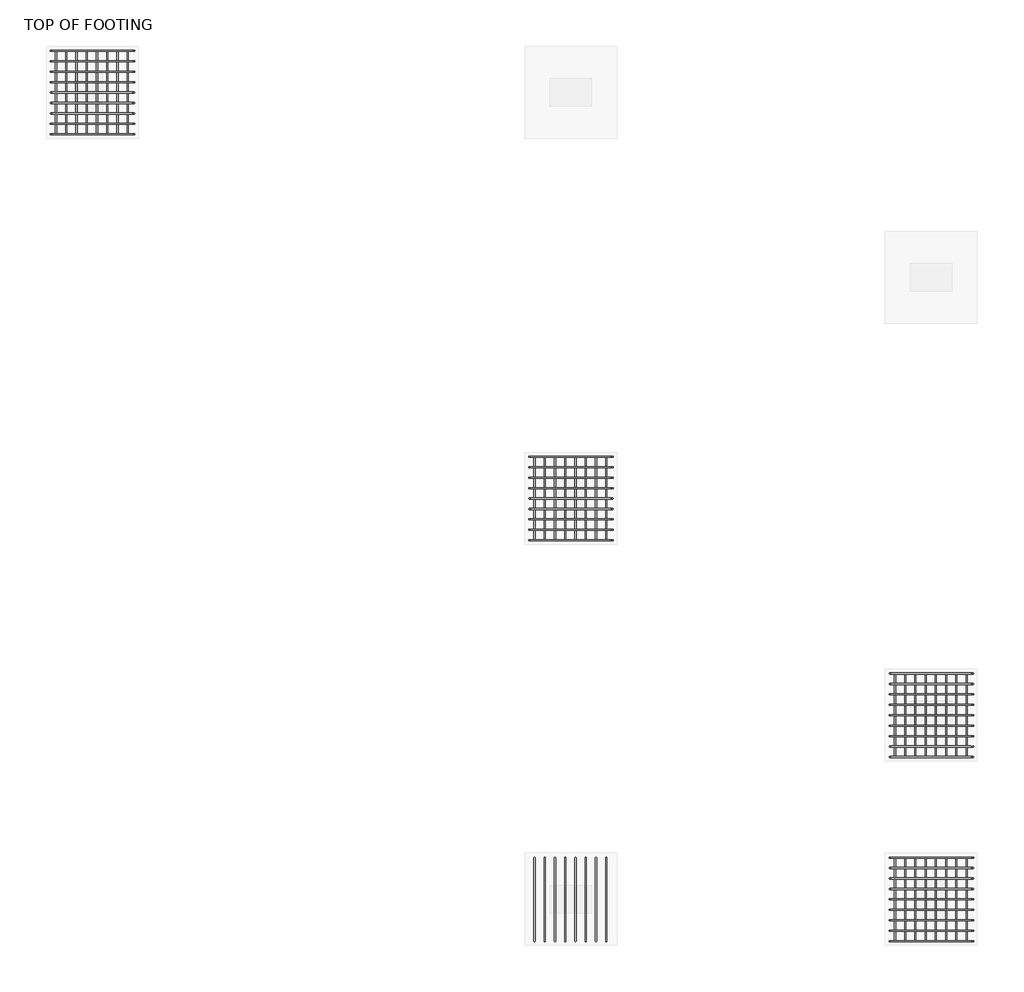
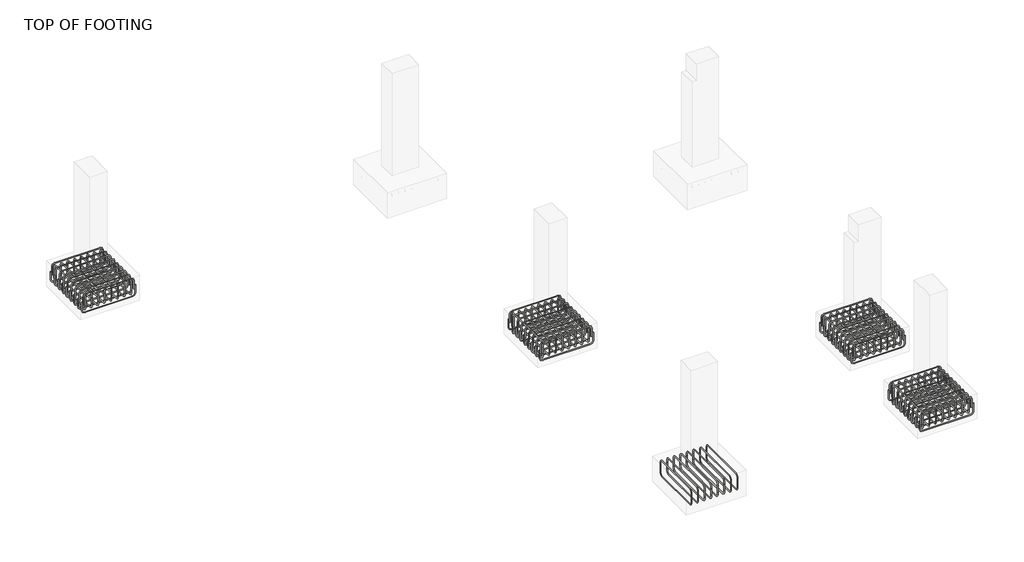
# One storey, part 4 of 20: 18 reinforcing bars.
"""IFC4 building model written with IfcOpenShell, lengths in millimetres."""

from ifc_helpers import new_model, si_unit, point, frame, origin, place, context, project, spatial, polyline, circle_curve, trimmed, segment, composite_curve, source, transform, mapped, element, save
from ifc_brep_helpers import swept_disk

model = new_model("IFC4")

# Units and contexts
model_context = context("Model", 3, world=origin())
ifc_project = project(units=[si_unit("LENGTHUNIT", "METRE", prefix="MILLI")], contexts=[model_context])

# Site, building, storey
site = spatial("IfcSite", under=ifc_project)
building = spatial("IfcBuilding", under=site)
storey = spatial("IfcBuildingStorey", under=building, Name="TOP OF FOOTING", Elevation=-1828.8)

# Reinforcing bars
placement = place(None, origin())
reinforcing_bar_shape = source(origin(), model_context, "Body", "SolidModel", [
    swept_disk(composite_curve([segment(polyline([(-10485.1605653, -2535.8035766, -2006.6587682), (-10485.1605653, -2535.8035766, -2153.9587682)]), True, "CONTINUOUS"), segment(trimmed(circle_curve(frame((-10531.5105653, -2535.8035766, -2153.9587682), z_axis=(0.0, 1.0, 0.0), x_axis=(46.349999999998545, 0.0, 0.0)), 46.35), [point((-10485.1605653, -2535.8035766, -2153.9587682))], [point((-10531.5105653, -2535.8035766, -2200.3087682))], True, "CARTESIAN"), True, "CONTINUOUS"), segment(polyline([(-10531.5105653, -2535.8035766, -2200.3087682), (-11346.1105653, -2535.8035766, -2200.3087682)]), True, "CONTINUOUS"), segment(trimmed(circle_curve(frame((-11346.1105653, -2535.8035766, -2153.9587682), z_axis=(0.0, 1.0, 0.0), x_axis=(0.0, 0.0, -46.34999999999991)), 46.35), [point((-11346.1105653, -2535.8035766, -2200.3087682))], [point((-11392.4605653, -2535.8035766, -2153.9587682))], True, "CARTESIAN"), True, "CONTINUOUS"), segment(polyline([(-11392.4605653, -2535.8035766, -2153.9587682), (-11392.4605653, -2535.8035766, -2006.6587682)]), True, "CONTINUOUS")], self_intersect=False), 6.35),
])
element("IfcReinforcingBar", 1, at=placement, inside=storey, context=model_context, shape_type="MappedRepresentation", body=[
    mapped(reinforcing_bar_shape, transform((0.0, 0.0, 0.0), x_axis=(1.0, 0.0, 0.0), y_axis=(0.0, 1.0, 0.0), z_axis=(0.0, 0.0, 1.0))),
    mapped(reinforcing_bar_shape, transform((0.0, -113.4125, 0.0), x_axis=(1.0, 0.0, 0.0), y_axis=(0.0, 1.0, 0.0), z_axis=(0.0, 0.0, 1.0))),
    mapped(reinforcing_bar_shape, transform((0.0, -226.825, 0.0), x_axis=(1.0, 0.0, 0.0), y_axis=(0.0, 1.0, 0.0), z_axis=(0.0, 0.0, 1.0))),
    mapped(reinforcing_bar_shape, transform((0.0, -340.2375, 0.0), x_axis=(1.0, 0.0, 0.0), y_axis=(0.0, 1.0, 0.0), z_axis=(0.0, 0.0, 1.0))),
    mapped(reinforcing_bar_shape, transform((0.0, -453.65, 0.0), x_axis=(1.0, 0.0, 0.0), y_axis=(0.0, 1.0, 0.0), z_axis=(0.0, 0.0, 1.0))),
    mapped(reinforcing_bar_shape, transform((0.0, -567.0625, 0.0), x_axis=(1.0, 0.0, 0.0), y_axis=(0.0, 1.0, 0.0), z_axis=(0.0, 0.0, 1.0))),
    mapped(reinforcing_bar_shape, transform((0.0, -680.475, 0.0), x_axis=(1.0, 0.0, 0.0), y_axis=(0.0, 1.0, 0.0), z_axis=(0.0, 0.0, 1.0))),
    mapped(reinforcing_bar_shape, transform((0.0, -793.8875, 0.0), x_axis=(1.0, 0.0, 0.0), y_axis=(0.0, 1.0, 0.0), z_axis=(0.0, 0.0, 1.0))),
    mapped(reinforcing_bar_shape, transform((0.0, -907.3, 0.0), x_axis=(1.0, 0.0, 0.0), y_axis=(0.0, 1.0, 0.0), z_axis=(0.0, 0.0, 1.0))),
])
reinforcing_bar_2_shape = source(origin(), model_context, "Body", "SolidModel", [
    swept_disk(composite_curve([segment(polyline([(-11372.986454, -2535.8035766, -2068.8), (-11372.986454, -2535.8035766, -1921.5)]), True, "CONTINUOUS"), segment(trimmed(circle_curve(frame((-11326.636454, -2535.8035766, -1921.5), z_axis=(0.0, 1.0, 0.0), x_axis=(-46.350000000000364, 0.0, 0.0)), 46.35), [point((-11372.986454, -2535.8035766, -1921.5))], [point((-11326.636454, -2535.8035766, -1875.15))], True, "CARTESIAN"), True, "CONTINUOUS"), segment(polyline([(-11326.636454, -2535.8035766, -1875.15), (-10557.1730543, -2535.8035766, -1875.15)]), True, "CONTINUOUS"), segment(trimmed(circle_curve(frame((-10557.1730543, -2535.8035766, -1921.5), z_axis=(0.0, 1.0, 0.0), x_axis=(0.0, 0.0, 46.34999999999991)), 46.35), [point((-10557.1730543, -2535.8035766, -1875.15))], [point((-10510.8230543, -2535.8035766, -1921.5))], True, "CARTESIAN"), True, "CONTINUOUS"), segment(polyline([(-10510.8230543, -2535.8035766, -1921.5), (-10510.8230543, -2535.8035766, -2068.8)]), True, "CONTINUOUS")], self_intersect=False), 6.35),
])
element("IfcReinforcingBar", 2, at=placement, inside=storey, context=model_context, shape_type="MappedRepresentation", body=[
    mapped(reinforcing_bar_2_shape, transform((0.0, 0.0, 0.0), x_axis=(1.0, 0.0, 0.0), y_axis=(0.0, 1.0, 0.0), z_axis=(0.0, 0.0, 1.0))),
    mapped(reinforcing_bar_2_shape, transform((0.0, -113.4125, 0.0), x_axis=(1.0, 0.0, 0.0), y_axis=(0.0, 1.0, 0.0), z_axis=(0.0, 0.0, 1.0))),
    mapped(reinforcing_bar_2_shape, transform((0.0, -226.825, 0.0), x_axis=(1.0, 0.0, 0.0), y_axis=(0.0, 1.0, 0.0), z_axis=(0.0, 0.0, 1.0))),
    mapped(reinforcing_bar_2_shape, transform((0.0, -340.2375, 0.0), x_axis=(1.0, 0.0, 0.0), y_axis=(0.0, 1.0, 0.0), z_axis=(0.0, 0.0, 1.0))),
    mapped(reinforcing_bar_2_shape, transform((0.0, -453.65, 0.0), x_axis=(1.0, 0.0, 0.0), y_axis=(0.0, 1.0, 0.0), z_axis=(0.0, 0.0, 1.0))),
    mapped(reinforcing_bar_2_shape, transform((0.0, -567.0625, 0.0), x_axis=(1.0, 0.0, 0.0), y_axis=(0.0, 1.0, 0.0), z_axis=(0.0, 0.0, 1.0))),
    mapped(reinforcing_bar_2_shape, transform((0.0, -680.475, 0.0), x_axis=(1.0, 0.0, 0.0), y_axis=(0.0, 1.0, 0.0), z_axis=(0.0, 0.0, 1.0))),
    mapped(reinforcing_bar_2_shape, transform((0.0, -793.8875, 0.0), x_axis=(1.0, 0.0, 0.0), y_axis=(0.0, 1.0, 0.0), z_axis=(0.0, 0.0, 1.0))),
    mapped(reinforcing_bar_2_shape, transform((0.0, -907.3, 0.0), x_axis=(1.0, 0.0, 0.0), y_axis=(0.0, 1.0, 0.0), z_axis=(0.0, 0.0, 1.0))),
])
reinforcing_bar_3_shape = source(origin(), model_context, "Body", "SolidModel", [
    swept_disk(composite_curve([segment(polyline([(-10556.6575267, -2535.8035766, -2086.1951968), (-10556.6575267, -2535.8035766, -1938.8951968)]), True, "CONTINUOUS"), segment(trimmed(circle_curve(frame((-10556.6575267, -2582.1535766, -1938.8951968), z_axis=(1.0, 0.0, 0.0), x_axis=(0.0, 46.350000000000364, 0.0)), 46.35), [point((-10556.6575267, -2535.8035766, -1938.8951968))], [point((-10556.6575267, -2582.1535766, -1892.5451968))], True, "CARTESIAN"), True, "CONTINUOUS"), segment(polyline([(-10556.6575267, -2582.1535766, -1892.5451968), (-10556.6575267, -3396.7535766, -1892.5451968)]), True, "CONTINUOUS"), segment(trimmed(circle_curve(frame((-10556.6575267, -3396.7535766, -1938.8951968), z_axis=(1.0, 0.0, 0.0), x_axis=(0.0, 0.0, 46.34999999999991)), 46.35), [point((-10556.6575267, -3396.7535766, -1892.5451968))], [point((-10556.6575267, -3443.1035766, -1938.8951968))], True, "CARTESIAN"), True, "CONTINUOUS"), segment(polyline([(-10556.6575267, -3443.1035766, -1938.8951968), (-10556.6575267, -3443.1035766, -2086.1951968)]), True, "CONTINUOUS")], self_intersect=False), 6.35),
])
element("IfcReinforcingBar", 3, at=placement, inside=storey, context=model_context, shape_type="MappedRepresentation", body=[
    mapped(reinforcing_bar_3_shape, transform((0.0, 0.0, 0.0), x_axis=(1.0, 0.0, 0.0), y_axis=(0.0, 1.0, 0.0), z_axis=(0.0, 0.0, 1.0))),
    mapped(reinforcing_bar_3_shape, transform((-111.2862402, 0.0, 0.0), x_axis=(1.0, 0.0, 0.0), y_axis=(0.0, 1.0, 0.0), z_axis=(0.0, 0.0, 1.0))),
    mapped(reinforcing_bar_3_shape, transform((-222.5724804, 0.0, 0.0), x_axis=(1.0, 0.0, 0.0), y_axis=(0.0, 1.0, 0.0), z_axis=(0.0, 0.0, 1.0))),
    mapped(reinforcing_bar_3_shape, transform((-333.8587205, 0.0, 0.0), x_axis=(1.0, 0.0, 0.0), y_axis=(0.0, 1.0, 0.0), z_axis=(0.0, 0.0, 1.0))),
    mapped(reinforcing_bar_3_shape, transform((-445.1449607, 0.0, 0.0), x_axis=(1.0, 0.0, 0.0), y_axis=(0.0, 1.0, 0.0), z_axis=(0.0, 0.0, 1.0))),
    mapped(reinforcing_bar_3_shape, transform((-556.4312009, 0.0, 0.0), x_axis=(1.0, 0.0, 0.0), y_axis=(0.0, 1.0, 0.0), z_axis=(0.0, 0.0, 1.0))),
    mapped(reinforcing_bar_3_shape, transform((-667.7174411, 0.0, 0.0), x_axis=(1.0, 0.0, 0.0), y_axis=(0.0, 1.0, 0.0), z_axis=(0.0, 0.0, 1.0))),
    mapped(reinforcing_bar_3_shape, transform((-779.0036813, 0.0, 0.0), x_axis=(1.0, 0.0, 0.0), y_axis=(0.0, 1.0, 0.0), z_axis=(0.0, 0.0, 1.0))),
])
reinforcing_bar_4_shape = source(origin(), model_context, "Body", "SolidModel", [
    swept_disk(composite_curve([segment(polyline([(-11335.661208, -2535.8035766, -1979.1645013), (-11335.661208, -2535.8035766, -2126.4645013)]), True, "CONTINUOUS"), segment(trimmed(circle_curve(frame((-11335.661208, -2582.1535766, -2126.4645013), z_axis=(-1.0, 0.0, 0.0), x_axis=(0.0, 46.350000000000364, 0.0)), 46.35), [point((-11335.661208, -2535.8035766, -2126.4645013))], [point((-11335.661208, -2582.1535766, -2172.8145013))], True, "CARTESIAN"), True, "CONTINUOUS"), segment(polyline([(-11335.661208, -2582.1535766, -2172.8145013), (-11335.661208, -3396.7535766, -2172.8145013)]), True, "CONTINUOUS"), segment(trimmed(circle_curve(frame((-11335.661208, -3396.7535766, -2126.4645013), z_axis=(-1.0, 0.0, 0.0), x_axis=(0.0, 0.0, -46.34999999999991)), 46.35), [point((-11335.661208, -3396.7535766, -2172.8145013))], [point((-11335.661208, -3443.1035766, -2126.4645013))], True, "CARTESIAN"), True, "CONTINUOUS"), segment(polyline([(-11335.661208, -3443.1035766, -2126.4645013), (-11335.661208, -3443.1035766, -1979.1645013)]), True, "CONTINUOUS")], self_intersect=False), 6.35),
])
element("IfcReinforcingBar", 4, at=placement, inside=storey, context=model_context, shape_type="MappedRepresentation", body=[
    mapped(reinforcing_bar_4_shape, transform((0.0, 0.0, 0.0), x_axis=(1.0, 0.0, 0.0), y_axis=(0.0, 1.0, 0.0), z_axis=(0.0, 0.0, 1.0))),
    mapped(reinforcing_bar_4_shape, transform((111.2862402, 0.0, 0.0), x_axis=(1.0, 0.0, 0.0), y_axis=(0.0, 1.0, 0.0), z_axis=(0.0, 0.0, 1.0))),
    mapped(reinforcing_bar_4_shape, transform((222.5724804, 0.0, 0.0), x_axis=(1.0, 0.0, 0.0), y_axis=(0.0, 1.0, 0.0), z_axis=(0.0, 0.0, 1.0))),
    mapped(reinforcing_bar_4_shape, transform((333.8587205, 0.0, 0.0), x_axis=(1.0, 0.0, 0.0), y_axis=(0.0, 1.0, 0.0), z_axis=(0.0, 0.0, 1.0))),
    mapped(reinforcing_bar_4_shape, transform((445.1449607, 0.0, 0.0), x_axis=(1.0, 0.0, 0.0), y_axis=(0.0, 1.0, 0.0), z_axis=(0.0, 0.0, 1.0))),
    mapped(reinforcing_bar_4_shape, transform((556.4312009, 0.0, 0.0), x_axis=(1.0, 0.0, 0.0), y_axis=(0.0, 1.0, 0.0), z_axis=(0.0, 0.0, 1.0))),
    mapped(reinforcing_bar_4_shape, transform((667.7174411, 0.0, 0.0), x_axis=(1.0, 0.0, 0.0), y_axis=(0.0, 1.0, 0.0), z_axis=(0.0, 0.0, 1.0))),
    mapped(reinforcing_bar_4_shape, transform((779.0036813, 0.0, 0.0), x_axis=(1.0, 0.0, 0.0), y_axis=(0.0, 1.0, 0.0), z_axis=(0.0, 0.0, 1.0))),
])
reinforcing_bar_5_shape = source(origin(), model_context, "Body", "SolidModel", [
    swept_disk(composite_curve([segment(polyline([(-5285.1605653, -6947.9729916, -2006.6587682), (-5285.1605653, -6947.9729916, -2153.9587682)]), True, "CONTINUOUS"), segment(trimmed(circle_curve(frame((-5331.5105653, -6947.9729916, -2153.9587682), z_axis=(0.0, 1.0, 0.0), x_axis=(46.350000000000364, 0.0, 0.0)), 46.35), [point((-5285.1605653, -6947.9729916, -2153.9587682))], [point((-5331.5105653, -6947.9729916, -2200.3087682))], True, "CARTESIAN"), True, "CONTINUOUS"), segment(polyline([(-5331.5105653, -6947.9729916, -2200.3087682), (-6146.1105653, -6947.9729916, -2200.3087682)]), True, "CONTINUOUS"), segment(trimmed(circle_curve(frame((-6146.1105653, -6947.9729916, -2153.9587682), z_axis=(0.0, 1.0, 0.0), x_axis=(0.0, 0.0, -46.34999999999991)), 46.35), [point((-6146.1105653, -6947.9729916, -2200.3087682))], [point((-6192.4605653, -6947.9729916, -2153.9587682))], True, "CARTESIAN"), True, "CONTINUOUS"), segment(polyline([(-6192.4605653, -6947.9729916, -2153.9587682), (-6192.4605653, -6947.9729916, -2006.6587682)]), True, "CONTINUOUS")], self_intersect=False), 6.35),
])
element("IfcReinforcingBar", 5, at=placement, inside=storey, context=model_context, shape_type="MappedRepresentation", body=[
    mapped(reinforcing_bar_5_shape, transform((0.0, 0.0, 0.0), x_axis=(1.0, 0.0, 0.0), y_axis=(0.0, 1.0, 0.0), z_axis=(0.0, 0.0, 1.0))),
    mapped(reinforcing_bar_5_shape, transform((0.0, -113.4125, 0.0), x_axis=(1.0, 0.0, 0.0), y_axis=(0.0, 1.0, 0.0), z_axis=(0.0, 0.0, 1.0))),
    mapped(reinforcing_bar_5_shape, transform((0.0, -226.825, 0.0), x_axis=(1.0, 0.0, 0.0), y_axis=(0.0, 1.0, 0.0), z_axis=(0.0, 0.0, 1.0))),
    mapped(reinforcing_bar_5_shape, transform((0.0, -340.2375, 0.0), x_axis=(1.0, 0.0, 0.0), y_axis=(0.0, 1.0, 0.0), z_axis=(0.0, 0.0, 1.0))),
    mapped(reinforcing_bar_5_shape, transform((0.0, -453.65, 0.0), x_axis=(1.0, 0.0, 0.0), y_axis=(0.0, 1.0, 0.0), z_axis=(0.0, 0.0, 1.0))),
    mapped(reinforcing_bar_5_shape, transform((0.0, -567.0625, 0.0), x_axis=(1.0, 0.0, 0.0), y_axis=(0.0, 1.0, 0.0), z_axis=(0.0, 0.0, 1.0))),
    mapped(reinforcing_bar_5_shape, transform((0.0, -680.475, 0.0), x_axis=(1.0, 0.0, 0.0), y_axis=(0.0, 1.0, 0.0), z_axis=(0.0, 0.0, 1.0))),
    mapped(reinforcing_bar_5_shape, transform((0.0, -793.8875, 0.0), x_axis=(1.0, 0.0, 0.0), y_axis=(0.0, 1.0, 0.0), z_axis=(0.0, 0.0, 1.0))),
    mapped(reinforcing_bar_5_shape, transform((0.0, -907.3, 0.0), x_axis=(1.0, 0.0, 0.0), y_axis=(0.0, 1.0, 0.0), z_axis=(0.0, 0.0, 1.0))),
])
reinforcing_bar_6_shape = source(origin(), model_context, "Body", "SolidModel", [
    swept_disk(composite_curve([segment(polyline([(-6172.986454, -6947.9729916, -2068.8), (-6172.986454, -6947.9729916, -1921.5)]), True, "CONTINUOUS"), segment(trimmed(circle_curve(frame((-6126.636454, -6947.9729916, -1921.5), z_axis=(0.0, 1.0, 0.0), x_axis=(-46.349999999999454, 0.0, 0.0)), 46.35), [point((-6172.986454, -6947.9729916, -1921.5))], [point((-6126.636454, -6947.9729916, -1875.15))], True, "CARTESIAN"), True, "CONTINUOUS"), segment(polyline([(-6126.636454, -6947.9729916, -1875.15), (-5357.1730543, -6947.9729916, -1875.15)]), True, "CONTINUOUS"), segment(trimmed(circle_curve(frame((-5357.1730543, -6947.9729916, -1921.5), z_axis=(0.0, 1.0, 0.0), x_axis=(0.0, 0.0, 46.34999999999991)), 46.35), [point((-5357.1730543, -6947.9729916, -1875.15))], [point((-5310.8230543, -6947.9729916, -1921.5))], True, "CARTESIAN"), True, "CONTINUOUS"), segment(polyline([(-5310.8230543, -6947.9729916, -1921.5), (-5310.8230543, -6947.9729916, -2068.8)]), True, "CONTINUOUS")], self_intersect=False), 6.35),
])
element("IfcReinforcingBar", 6, at=placement, inside=storey, context=model_context, shape_type="MappedRepresentation", body=[
    mapped(reinforcing_bar_6_shape, transform((0.0, 0.0, 0.0), x_axis=(1.0, 0.0, 0.0), y_axis=(0.0, 1.0, 0.0), z_axis=(0.0, 0.0, 1.0))),
    mapped(reinforcing_bar_6_shape, transform((0.0, -113.4125, 0.0), x_axis=(1.0, 0.0, 0.0), y_axis=(0.0, 1.0, 0.0), z_axis=(0.0, 0.0, 1.0))),
    mapped(reinforcing_bar_6_shape, transform((0.0, -226.825, 0.0), x_axis=(1.0, 0.0, 0.0), y_axis=(0.0, 1.0, 0.0), z_axis=(0.0, 0.0, 1.0))),
    mapped(reinforcing_bar_6_shape, transform((0.0, -340.2375, 0.0), x_axis=(1.0, 0.0, 0.0), y_axis=(0.0, 1.0, 0.0), z_axis=(0.0, 0.0, 1.0))),
    mapped(reinforcing_bar_6_shape, transform((0.0, -453.65, 0.0), x_axis=(1.0, 0.0, 0.0), y_axis=(0.0, 1.0, 0.0), z_axis=(0.0, 0.0, 1.0))),
    mapped(reinforcing_bar_6_shape, transform((0.0, -567.0625, 0.0), x_axis=(1.0, 0.0, 0.0), y_axis=(0.0, 1.0, 0.0), z_axis=(0.0, 0.0, 1.0))),
    mapped(reinforcing_bar_6_shape, transform((0.0, -680.475, 0.0), x_axis=(1.0, 0.0, 0.0), y_axis=(0.0, 1.0, 0.0), z_axis=(0.0, 0.0, 1.0))),
    mapped(reinforcing_bar_6_shape, transform((0.0, -793.8875, 0.0), x_axis=(1.0, 0.0, 0.0), y_axis=(0.0, 1.0, 0.0), z_axis=(0.0, 0.0, 1.0))),
    mapped(reinforcing_bar_6_shape, transform((0.0, -907.3, 0.0), x_axis=(1.0, 0.0, 0.0), y_axis=(0.0, 1.0, 0.0), z_axis=(0.0, 0.0, 1.0))),
])
reinforcing_bar_7_shape = source(origin(), model_context, "Body", "SolidModel", [
    swept_disk(composite_curve([segment(polyline([(-5356.6575267, -6947.9729916, -2086.1951968), (-5356.6575267, -6947.9729916, -1938.8951968)]), True, "CONTINUOUS"), segment(trimmed(circle_curve(frame((-5356.6575267, -6994.3229916, -1938.8951968), z_axis=(1.0, 0.0, 0.0), x_axis=(0.0, 46.350000000000364, 0.0)), 46.35), [point((-5356.6575267, -6947.9729916, -1938.8951968))], [point((-5356.6575267, -6994.3229916, -1892.5451968))], True, "CARTESIAN"), True, "CONTINUOUS"), segment(polyline([(-5356.6575267, -6994.3229916, -1892.5451968), (-5356.6575267, -7808.9229916, -1892.5451968)]), True, "CONTINUOUS"), segment(trimmed(circle_curve(frame((-5356.6575267, -7808.9229916, -1938.8951968), z_axis=(1.0, 0.0, 0.0), x_axis=(0.0, 0.0, 46.34999999999991)), 46.35), [point((-5356.6575267, -7808.9229916, -1892.5451968))], [point((-5356.6575267, -7855.2729916, -1938.8951968))], True, "CARTESIAN"), True, "CONTINUOUS"), segment(polyline([(-5356.6575267, -7855.2729916, -1938.8951968), (-5356.6575267, -7855.2729916, -2086.1951968)]), True, "CONTINUOUS")], self_intersect=False), 6.35),
])
element("IfcReinforcingBar", 7, at=placement, inside=storey, context=model_context, shape_type="MappedRepresentation", body=[
    mapped(reinforcing_bar_7_shape, transform((0.0, 0.0, 0.0), x_axis=(1.0, 0.0, 0.0), y_axis=(0.0, 1.0, 0.0), z_axis=(0.0, 0.0, 1.0))),
    mapped(reinforcing_bar_7_shape, transform((-111.2862402, 0.0, 0.0), x_axis=(1.0, 0.0, 0.0), y_axis=(0.0, 1.0, 0.0), z_axis=(0.0, 0.0, 1.0))),
    mapped(reinforcing_bar_7_shape, transform((-222.5724804, 0.0, 0.0), x_axis=(1.0, 0.0, 0.0), y_axis=(0.0, 1.0, 0.0), z_axis=(0.0, 0.0, 1.0))),
    mapped(reinforcing_bar_7_shape, transform((-333.8587205, 0.0, 0.0), x_axis=(1.0, 0.0, 0.0), y_axis=(0.0, 1.0, 0.0), z_axis=(0.0, 0.0, 1.0))),
    mapped(reinforcing_bar_7_shape, transform((-445.1449607, 0.0, 0.0), x_axis=(1.0, 0.0, 0.0), y_axis=(0.0, 1.0, 0.0), z_axis=(0.0, 0.0, 1.0))),
    mapped(reinforcing_bar_7_shape, transform((-556.4312009, 0.0, 0.0), x_axis=(1.0, 0.0, 0.0), y_axis=(0.0, 1.0, 0.0), z_axis=(0.0, 0.0, 1.0))),
    mapped(reinforcing_bar_7_shape, transform((-667.7174411, 0.0, 0.0), x_axis=(1.0, 0.0, 0.0), y_axis=(0.0, 1.0, 0.0), z_axis=(0.0, 0.0, 1.0))),
    mapped(reinforcing_bar_7_shape, transform((-779.0036813, 0.0, 0.0), x_axis=(1.0, 0.0, 0.0), y_axis=(0.0, 1.0, 0.0), z_axis=(0.0, 0.0, 1.0))),
])
reinforcing_bar_8_shape = source(origin(), model_context, "Body", "SolidModel", [
    swept_disk(composite_curve([segment(polyline([(-6135.661208, -6947.9729916, -1979.1645013), (-6135.661208, -6947.9729916, -2126.4645013)]), True, "CONTINUOUS"), segment(trimmed(circle_curve(frame((-6135.661208, -6994.3229916, -2126.4645013), z_axis=(-1.0, 0.0, 0.0), x_axis=(0.0, 46.350000000000364, 0.0)), 46.35), [point((-6135.661208, -6947.9729916, -2126.4645013))], [point((-6135.661208, -6994.3229916, -2172.8145013))], True, "CARTESIAN"), True, "CONTINUOUS"), segment(polyline([(-6135.661208, -6994.3229916, -2172.8145013), (-6135.661208, -7808.9229916, -2172.8145013)]), True, "CONTINUOUS"), segment(trimmed(circle_curve(frame((-6135.661208, -7808.9229916, -2126.4645013), z_axis=(-1.0, 0.0, 0.0), x_axis=(0.0, 0.0, -46.34999999999991)), 46.35), [point((-6135.661208, -7808.9229916, -2172.8145013))], [point((-6135.661208, -7855.2729916, -2126.4645013))], True, "CARTESIAN"), True, "CONTINUOUS"), segment(polyline([(-6135.661208, -7855.2729916, -2126.4645013), (-6135.661208, -7855.2729916, -1979.1645013)]), True, "CONTINUOUS")], self_intersect=False), 6.35),
])
element("IfcReinforcingBar", 8, at=placement, inside=storey, context=model_context, shape_type="MappedRepresentation", body=[
    mapped(reinforcing_bar_8_shape, transform((0.0, 0.0, 0.0), x_axis=(1.0, 0.0, 0.0), y_axis=(0.0, 1.0, 0.0), z_axis=(0.0, 0.0, 1.0))),
    mapped(reinforcing_bar_8_shape, transform((111.2862402, 0.0, 0.0), x_axis=(1.0, 0.0, 0.0), y_axis=(0.0, 1.0, 0.0), z_axis=(0.0, 0.0, 1.0))),
    mapped(reinforcing_bar_8_shape, transform((222.5724804, 0.0, 0.0), x_axis=(1.0, 0.0, 0.0), y_axis=(0.0, 1.0, 0.0), z_axis=(0.0, 0.0, 1.0))),
    mapped(reinforcing_bar_8_shape, transform((333.8587205, 0.0, 0.0), x_axis=(1.0, 0.0, 0.0), y_axis=(0.0, 1.0, 0.0), z_axis=(0.0, 0.0, 1.0))),
    mapped(reinforcing_bar_8_shape, transform((445.1449607, 0.0, 0.0), x_axis=(1.0, 0.0, 0.0), y_axis=(0.0, 1.0, 0.0), z_axis=(0.0, 0.0, 1.0))),
    mapped(reinforcing_bar_8_shape, transform((556.4312009, 0.0, 0.0), x_axis=(1.0, 0.0, 0.0), y_axis=(0.0, 1.0, 0.0), z_axis=(0.0, 0.0, 1.0))),
    mapped(reinforcing_bar_8_shape, transform((667.7174411, 0.0, 0.0), x_axis=(1.0, 0.0, 0.0), y_axis=(0.0, 1.0, 0.0), z_axis=(0.0, 0.0, 1.0))),
    mapped(reinforcing_bar_8_shape, transform((779.0036813, 0.0, 0.0), x_axis=(1.0, 0.0, 0.0), y_axis=(0.0, 1.0, 0.0), z_axis=(0.0, 0.0, 1.0))),
])
reinforcing_bar_9_shape = source(origin(), model_context, "Body", "SolidModel", [
    swept_disk(composite_curve([segment(polyline([(-5356.6575267, -11304.2470059, -2086.1951968), (-5356.6575267, -11304.2470059, -1938.8951968)]), True, "CONTINUOUS"), segment(trimmed(circle_curve(frame((-5356.6575267, -11350.5970059, -1938.8951968), z_axis=(1.0, 0.0, 0.0), x_axis=(0.0, 46.349999999998545, 0.0)), 46.35), [point((-5356.6575267, -11304.2470059, -1938.8951968))], [point((-5356.6575267, -11350.5970059, -1892.5451968))], True, "CARTESIAN"), True, "CONTINUOUS"), segment(polyline([(-5356.6575267, -11350.5970059, -1892.5451968), (-5356.6575267, -12165.1970059, -1892.5451968)]), True, "CONTINUOUS"), segment(trimmed(circle_curve(frame((-5356.6575267, -12165.1970059, -1938.8951968), z_axis=(1.0, 0.0, 0.0), x_axis=(0.0, 0.0, 46.34999999999991)), 46.35), [point((-5356.6575267, -12165.1970059, -1892.5451968))], [point((-5356.6575267, -12211.5470059, -1938.8951968))], True, "CARTESIAN"), True, "CONTINUOUS"), segment(polyline([(-5356.6575267, -12211.5470059, -1938.8951968), (-5356.6575267, -12211.5470059, -2086.1951968)]), True, "CONTINUOUS")], self_intersect=False), 6.35),
])
element("IfcReinforcingBar", 9, at=placement, inside=storey, context=model_context, shape_type="MappedRepresentation", body=[
    mapped(reinforcing_bar_9_shape, transform((0.0, 0.0, 0.0), x_axis=(1.0, 0.0, 0.0), y_axis=(0.0, 1.0, 0.0), z_axis=(0.0, 0.0, 1.0))),
    mapped(reinforcing_bar_9_shape, transform((-111.2862402, 0.0, 0.0), x_axis=(1.0, 0.0, 0.0), y_axis=(0.0, 1.0, 0.0), z_axis=(0.0, 0.0, 1.0))),
    mapped(reinforcing_bar_9_shape, transform((-222.5724804, 0.0, 0.0), x_axis=(1.0, 0.0, 0.0), y_axis=(0.0, 1.0, 0.0), z_axis=(0.0, 0.0, 1.0))),
    mapped(reinforcing_bar_9_shape, transform((-333.8587205, 0.0, 0.0), x_axis=(1.0, 0.0, 0.0), y_axis=(0.0, 1.0, 0.0), z_axis=(0.0, 0.0, 1.0))),
    mapped(reinforcing_bar_9_shape, transform((-445.1449607, 0.0, 0.0), x_axis=(1.0, 0.0, 0.0), y_axis=(0.0, 1.0, 0.0), z_axis=(0.0, 0.0, 1.0))),
    mapped(reinforcing_bar_9_shape, transform((-556.4312009, 0.0, 0.0), x_axis=(1.0, 0.0, 0.0), y_axis=(0.0, 1.0, 0.0), z_axis=(0.0, 0.0, 1.0))),
    mapped(reinforcing_bar_9_shape, transform((-667.7174411, 0.0, 0.0), x_axis=(1.0, 0.0, 0.0), y_axis=(0.0, 1.0, 0.0), z_axis=(0.0, 0.0, 1.0))),
    mapped(reinforcing_bar_9_shape, transform((-779.0036813, 0.0, 0.0), x_axis=(1.0, 0.0, 0.0), y_axis=(0.0, 1.0, 0.0), z_axis=(0.0, 0.0, 1.0))),
])
reinforcing_bar_10_shape = source(origin(), model_context, "Body", "SolidModel", [
    swept_disk(composite_curve([segment(polyline([(-6135.661208, -11304.2470059, -1979.1645013), (-6135.661208, -11304.2470059, -2126.4645013)]), True, "CONTINUOUS"), segment(trimmed(circle_curve(frame((-6135.661208, -11350.5970059, -2126.4645013), z_axis=(-1.0, 0.0, 0.0), x_axis=(0.0, 46.349999999998545, 0.0)), 46.35), [point((-6135.661208, -11304.2470059, -2126.4645013))], [point((-6135.661208, -11350.5970059, -2172.8145013))], True, "CARTESIAN"), True, "CONTINUOUS"), segment(polyline([(-6135.661208, -11350.5970059, -2172.8145013), (-6135.661208, -12165.1970059, -2172.8145013)]), True, "CONTINUOUS"), segment(trimmed(circle_curve(frame((-6135.661208, -12165.1970059, -2126.4645013), z_axis=(-1.0, 0.0, 0.0), x_axis=(0.0, 0.0, -46.34999999999991)), 46.35), [point((-6135.661208, -12165.1970059, -2172.8145013))], [point((-6135.661208, -12211.5470059, -2126.4645013))], True, "CARTESIAN"), True, "CONTINUOUS"), segment(polyline([(-6135.661208, -12211.5470059, -2126.4645013), (-6135.661208, -12211.5470059, -1979.1645013)]), True, "CONTINUOUS")], self_intersect=False), 6.35),
])
element("IfcReinforcingBar", 10, at=placement, inside=storey, context=model_context, shape_type="MappedRepresentation", body=[
    mapped(reinforcing_bar_10_shape, transform((0.0, 0.0, 0.0), x_axis=(1.0, 0.0, 0.0), y_axis=(0.0, 1.0, 0.0), z_axis=(0.0, 0.0, 1.0))),
    mapped(reinforcing_bar_10_shape, transform((111.2862402, 0.0, 0.0), x_axis=(1.0, 0.0, 0.0), y_axis=(0.0, 1.0, 0.0), z_axis=(0.0, 0.0, 1.0))),
    mapped(reinforcing_bar_10_shape, transform((222.5724804, 0.0, 0.0), x_axis=(1.0, 0.0, 0.0), y_axis=(0.0, 1.0, 0.0), z_axis=(0.0, 0.0, 1.0))),
    mapped(reinforcing_bar_10_shape, transform((333.8587205, 0.0, 0.0), x_axis=(1.0, 0.0, 0.0), y_axis=(0.0, 1.0, 0.0), z_axis=(0.0, 0.0, 1.0))),
    mapped(reinforcing_bar_10_shape, transform((445.1449607, 0.0, 0.0), x_axis=(1.0, 0.0, 0.0), y_axis=(0.0, 1.0, 0.0), z_axis=(0.0, 0.0, 1.0))),
    mapped(reinforcing_bar_10_shape, transform((556.4312009, 0.0, 0.0), x_axis=(1.0, 0.0, 0.0), y_axis=(0.0, 1.0, 0.0), z_axis=(0.0, 0.0, 1.0))),
    mapped(reinforcing_bar_10_shape, transform((667.7174411, 0.0, 0.0), x_axis=(1.0, 0.0, 0.0), y_axis=(0.0, 1.0, 0.0), z_axis=(0.0, 0.0, 1.0))),
    mapped(reinforcing_bar_10_shape, transform((779.0036813, 0.0, 0.0), x_axis=(1.0, 0.0, 0.0), y_axis=(0.0, 1.0, 0.0), z_axis=(0.0, 0.0, 1.0))),
])
reinforcing_bar_11_shape = source(origin(), model_context, "Body", "SolidModel", [
    swept_disk(composite_curve([segment(polyline([(-1368.1365686, -11304.2470059, -2006.6587682), (-1368.1365686, -11304.2470059, -2153.9587682)]), True, "CONTINUOUS"), segment(trimmed(circle_curve(frame((-1414.4865686, -11304.2470059, -2153.9587682), z_axis=(0.0, 1.0, 0.0), x_axis=(46.350000000000136, 0.0, 0.0)), 46.35), [point((-1368.1365686, -11304.2470059, -2153.9587682))], [point((-1414.4865686, -11304.2470059, -2200.3087682))], True, "CARTESIAN"), True, "CONTINUOUS"), segment(polyline([(-1414.4865686, -11304.2470059, -2200.3087682), (-2229.0865686, -11304.2470059, -2200.3087682)]), True, "CONTINUOUS"), segment(trimmed(circle_curve(frame((-2229.0865686, -11304.2470059, -2153.9587682), z_axis=(0.0, 1.0, 0.0), x_axis=(0.0, 0.0, -46.34999999999991)), 46.35), [point((-2229.0865686, -11304.2470059, -2200.3087682))], [point((-2275.4365686, -11304.2470059, -2153.9587682))], True, "CARTESIAN"), True, "CONTINUOUS"), segment(polyline([(-2275.4365686, -11304.2470059, -2153.9587682), (-2275.4365686, -11304.2470059, -2006.6587682)]), True, "CONTINUOUS")], self_intersect=False), 6.35),
])
element("IfcReinforcingBar", 11, at=placement, inside=storey, context=model_context, shape_type="MappedRepresentation", body=[
    mapped(reinforcing_bar_11_shape, transform((0.0, 0.0, 0.0), x_axis=(1.0, 0.0, 0.0), y_axis=(0.0, 1.0, 0.0), z_axis=(0.0, 0.0, 1.0))),
    mapped(reinforcing_bar_11_shape, transform((0.0, -113.4125, 0.0), x_axis=(1.0, 0.0, 0.0), y_axis=(0.0, 1.0, 0.0), z_axis=(0.0, 0.0, 1.0))),
    mapped(reinforcing_bar_11_shape, transform((0.0, -226.825, 0.0), x_axis=(1.0, 0.0, 0.0), y_axis=(0.0, 1.0, 0.0), z_axis=(0.0, 0.0, 1.0))),
    mapped(reinforcing_bar_11_shape, transform((0.0, -340.2375, 0.0), x_axis=(1.0, 0.0, 0.0), y_axis=(0.0, 1.0, 0.0), z_axis=(0.0, 0.0, 1.0))),
    mapped(reinforcing_bar_11_shape, transform((0.0, -453.65, 0.0), x_axis=(1.0, 0.0, 0.0), y_axis=(0.0, 1.0, 0.0), z_axis=(0.0, 0.0, 1.0))),
    mapped(reinforcing_bar_11_shape, transform((0.0, -567.0625, 0.0), x_axis=(1.0, 0.0, 0.0), y_axis=(0.0, 1.0, 0.0), z_axis=(0.0, 0.0, 1.0))),
    mapped(reinforcing_bar_11_shape, transform((0.0, -680.475, 0.0), x_axis=(1.0, 0.0, 0.0), y_axis=(0.0, 1.0, 0.0), z_axis=(0.0, 0.0, 1.0))),
    mapped(reinforcing_bar_11_shape, transform((0.0, -793.8875, 0.0), x_axis=(1.0, 0.0, 0.0), y_axis=(0.0, 1.0, 0.0), z_axis=(0.0, 0.0, 1.0))),
    mapped(reinforcing_bar_11_shape, transform((0.0, -907.3, 0.0), x_axis=(1.0, 0.0, 0.0), y_axis=(0.0, 1.0, 0.0), z_axis=(0.0, 0.0, 1.0))),
])
reinforcing_bar_12_shape = source(origin(), model_context, "Body", "SolidModel", [
    swept_disk(composite_curve([segment(polyline([(-2255.9624573, -11304.2470059, -2068.8), (-2255.9624573, -11304.2470059, -1921.5)]), True, "CONTINUOUS"), segment(trimmed(circle_curve(frame((-2209.6124573, -11304.2470059, -1921.5), z_axis=(0.0, 1.0, 0.0), x_axis=(-46.34999999999991, 0.0, 0.0)), 46.35), [point((-2255.9624573, -11304.2470059, -1921.5))], [point((-2209.6124573, -11304.2470059, -1875.15))], True, "CARTESIAN"), True, "CONTINUOUS"), segment(polyline([(-2209.6124573, -11304.2470059, -1875.15), (-1440.1490576, -11304.2470059, -1875.15)]), True, "CONTINUOUS"), segment(trimmed(circle_curve(frame((-1440.1490576, -11304.2470059, -1921.5), z_axis=(0.0, 1.0, 0.0), x_axis=(0.0, 0.0, 46.34999999999991)), 46.35), [point((-1440.1490576, -11304.2470059, -1875.15))], [point((-1393.7990576, -11304.2470059, -1921.5))], True, "CARTESIAN"), True, "CONTINUOUS"), segment(polyline([(-1393.7990576, -11304.2470059, -1921.5), (-1393.7990576, -11304.2470059, -2068.8)]), True, "CONTINUOUS")], self_intersect=False), 6.35),
])
element("IfcReinforcingBar", 12, at=placement, inside=storey, context=model_context, shape_type="MappedRepresentation", body=[
    mapped(reinforcing_bar_12_shape, transform((0.0, 0.0, 0.0), x_axis=(1.0, 0.0, 0.0), y_axis=(0.0, 1.0, 0.0), z_axis=(0.0, 0.0, 1.0))),
    mapped(reinforcing_bar_12_shape, transform((0.0, -113.4125, 0.0), x_axis=(1.0, 0.0, 0.0), y_axis=(0.0, 1.0, 0.0), z_axis=(0.0, 0.0, 1.0))),
    mapped(reinforcing_bar_12_shape, transform((0.0, -226.825, 0.0), x_axis=(1.0, 0.0, 0.0), y_axis=(0.0, 1.0, 0.0), z_axis=(0.0, 0.0, 1.0))),
    mapped(reinforcing_bar_12_shape, transform((0.0, -340.2375, 0.0), x_axis=(1.0, 0.0, 0.0), y_axis=(0.0, 1.0, 0.0), z_axis=(0.0, 0.0, 1.0))),
    mapped(reinforcing_bar_12_shape, transform((0.0, -453.65, 0.0), x_axis=(1.0, 0.0, 0.0), y_axis=(0.0, 1.0, 0.0), z_axis=(0.0, 0.0, 1.0))),
    mapped(reinforcing_bar_12_shape, transform((0.0, -567.0625, 0.0), x_axis=(1.0, 0.0, 0.0), y_axis=(0.0, 1.0, 0.0), z_axis=(0.0, 0.0, 1.0))),
    mapped(reinforcing_bar_12_shape, transform((0.0, -680.475, 0.0), x_axis=(1.0, 0.0, 0.0), y_axis=(0.0, 1.0, 0.0), z_axis=(0.0, 0.0, 1.0))),
    mapped(reinforcing_bar_12_shape, transform((0.0, -793.8875, 0.0), x_axis=(1.0, 0.0, 0.0), y_axis=(0.0, 1.0, 0.0), z_axis=(0.0, 0.0, 1.0))),
    mapped(reinforcing_bar_12_shape, transform((0.0, -907.3, 0.0), x_axis=(1.0, 0.0, 0.0), y_axis=(0.0, 1.0, 0.0), z_axis=(0.0, 0.0, 1.0))),
])
reinforcing_bar_13_shape = source(origin(), model_context, "Body", "SolidModel", [
    swept_disk(composite_curve([segment(polyline([(-1439.63353, -11304.2470059, -2086.1951968), (-1439.63353, -11304.2470059, -1938.8951968)]), True, "CONTINUOUS"), segment(trimmed(circle_curve(frame((-1439.63353, -11350.5970059, -1938.8951968), z_axis=(1.0, 0.0, 0.0), x_axis=(0.0, 46.349999999998545, 0.0)), 46.35), [point((-1439.63353, -11304.2470059, -1938.8951968))], [point((-1439.63353, -11350.5970059, -1892.5451968))], True, "CARTESIAN"), True, "CONTINUOUS"), segment(polyline([(-1439.63353, -11350.5970059, -1892.5451968), (-1439.63353, -12165.1970059, -1892.5451968)]), True, "CONTINUOUS"), segment(trimmed(circle_curve(frame((-1439.63353, -12165.1970059, -1938.8951968), z_axis=(1.0, 0.0, 0.0), x_axis=(0.0, 0.0, 46.34999999999991)), 46.35), [point((-1439.63353, -12165.1970059, -1892.5451968))], [point((-1439.63353, -12211.5470059, -1938.8951968))], True, "CARTESIAN"), True, "CONTINUOUS"), segment(polyline([(-1439.63353, -12211.5470059, -1938.8951968), (-1439.63353, -12211.5470059, -2086.1951968)]), True, "CONTINUOUS")], self_intersect=False), 6.35),
])
element("IfcReinforcingBar", 13, at=placement, inside=storey, context=model_context, shape_type="MappedRepresentation", body=[
    mapped(reinforcing_bar_13_shape, transform((0.0, 0.0, 0.0), x_axis=(1.0, 0.0, 0.0), y_axis=(0.0, 1.0, 0.0), z_axis=(0.0, 0.0, 1.0))),
    mapped(reinforcing_bar_13_shape, transform((-111.2862402, 0.0, 0.0), x_axis=(1.0, 0.0, 0.0), y_axis=(0.0, 1.0, 0.0), z_axis=(0.0, 0.0, 1.0))),
    mapped(reinforcing_bar_13_shape, transform((-222.5724804, 0.0, 0.0), x_axis=(1.0, 0.0, 0.0), y_axis=(0.0, 1.0, 0.0), z_axis=(0.0, 0.0, 1.0))),
    mapped(reinforcing_bar_13_shape, transform((-333.8587205, 0.0, 0.0), x_axis=(1.0, 0.0, 0.0), y_axis=(0.0, 1.0, 0.0), z_axis=(0.0, 0.0, 1.0))),
    mapped(reinforcing_bar_13_shape, transform((-445.1449607, 0.0, 0.0), x_axis=(1.0, 0.0, 0.0), y_axis=(0.0, 1.0, 0.0), z_axis=(0.0, 0.0, 1.0))),
    mapped(reinforcing_bar_13_shape, transform((-556.4312009, 0.0, 0.0), x_axis=(1.0, 0.0, 0.0), y_axis=(0.0, 1.0, 0.0), z_axis=(0.0, 0.0, 1.0))),
    mapped(reinforcing_bar_13_shape, transform((-667.7174411, 0.0, 0.0), x_axis=(1.0, 0.0, 0.0), y_axis=(0.0, 1.0, 0.0), z_axis=(0.0, 0.0, 1.0))),
    mapped(reinforcing_bar_13_shape, transform((-779.0036813, 0.0, 0.0), x_axis=(1.0, 0.0, 0.0), y_axis=(0.0, 1.0, 0.0), z_axis=(0.0, 0.0, 1.0))),
])
reinforcing_bar_14_shape = source(origin(), model_context, "Body", "SolidModel", [
    swept_disk(composite_curve([segment(polyline([(-2218.6372113, -11304.2470059, -1979.1645013), (-2218.6372113, -11304.2470059, -2126.4645013)]), True, "CONTINUOUS"), segment(trimmed(circle_curve(frame((-2218.6372113, -11350.5970059, -2126.4645013), z_axis=(-1.0, 0.0, 0.0), x_axis=(0.0, 46.349999999998545, 0.0)), 46.35), [point((-2218.6372113, -11304.2470059, -2126.4645013))], [point((-2218.6372113, -11350.5970059, -2172.8145013))], True, "CARTESIAN"), True, "CONTINUOUS"), segment(polyline([(-2218.6372113, -11350.5970059, -2172.8145013), (-2218.6372113, -12165.1970059, -2172.8145013)]), True, "CONTINUOUS"), segment(trimmed(circle_curve(frame((-2218.6372113, -12165.1970059, -2126.4645013), z_axis=(-1.0, 0.0, 0.0), x_axis=(0.0, 0.0, -46.34999999999991)), 46.35), [point((-2218.6372113, -12165.1970059, -2172.8145013))], [point((-2218.6372113, -12211.5470059, -2126.4645013))], True, "CARTESIAN"), True, "CONTINUOUS"), segment(polyline([(-2218.6372113, -12211.5470059, -2126.4645013), (-2218.6372113, -12211.5470059, -1979.1645013)]), True, "CONTINUOUS")], self_intersect=False), 6.35),
])
element("IfcReinforcingBar", 14, at=placement, inside=storey, context=model_context, shape_type="MappedRepresentation", body=[
    mapped(reinforcing_bar_14_shape, transform((0.0, 0.0, 0.0), x_axis=(1.0, 0.0, 0.0), y_axis=(0.0, 1.0, 0.0), z_axis=(0.0, 0.0, 1.0))),
    mapped(reinforcing_bar_14_shape, transform((111.2862402, 0.0, 0.0), x_axis=(1.0, 0.0, 0.0), y_axis=(0.0, 1.0, 0.0), z_axis=(0.0, 0.0, 1.0))),
    mapped(reinforcing_bar_14_shape, transform((222.5724804, 0.0, 0.0), x_axis=(1.0, 0.0, 0.0), y_axis=(0.0, 1.0, 0.0), z_axis=(0.0, 0.0, 1.0))),
    mapped(reinforcing_bar_14_shape, transform((333.8587205, 0.0, 0.0), x_axis=(1.0, 0.0, 0.0), y_axis=(0.0, 1.0, 0.0), z_axis=(0.0, 0.0, 1.0))),
    mapped(reinforcing_bar_14_shape, transform((445.1449607, 0.0, 0.0), x_axis=(1.0, 0.0, 0.0), y_axis=(0.0, 1.0, 0.0), z_axis=(0.0, 0.0, 1.0))),
    mapped(reinforcing_bar_14_shape, transform((556.4312009, 0.0, 0.0), x_axis=(1.0, 0.0, 0.0), y_axis=(0.0, 1.0, 0.0), z_axis=(0.0, 0.0, 1.0))),
    mapped(reinforcing_bar_14_shape, transform((667.7174411, 0.0, 0.0), x_axis=(1.0, 0.0, 0.0), y_axis=(0.0, 1.0, 0.0), z_axis=(0.0, 0.0, 1.0))),
    mapped(reinforcing_bar_14_shape, transform((779.0036813, 0.0, 0.0), x_axis=(1.0, 0.0, 0.0), y_axis=(0.0, 1.0, 0.0), z_axis=(0.0, 0.0, 1.0))),
])
reinforcing_bar_15_shape = source(origin(), model_context, "Body", "SolidModel", [
    swept_disk(composite_curve([segment(polyline([(-1368.1365686, -9303.4578267, -2006.6587682), (-1368.1365686, -9303.4578267, -2153.9587682)]), True, "CONTINUOUS"), segment(trimmed(circle_curve(frame((-1414.4865686, -9303.4578267, -2153.9587682), z_axis=(0.0, 1.0, 0.0), x_axis=(46.350000000000136, 0.0, 0.0)), 46.35), [point((-1368.1365686, -9303.4578267, -2153.9587682))], [point((-1414.4865686, -9303.4578267, -2200.3087682))], True, "CARTESIAN"), True, "CONTINUOUS"), segment(polyline([(-1414.4865686, -9303.4578267, -2200.3087682), (-2229.0865686, -9303.4578267, -2200.3087682)]), True, "CONTINUOUS"), segment(trimmed(circle_curve(frame((-2229.0865686, -9303.4578267, -2153.9587682), z_axis=(0.0, 1.0, 0.0), x_axis=(0.0, 0.0, -46.34999999999991)), 46.35), [point((-2229.0865686, -9303.4578267, -2200.3087682))], [point((-2275.4365686, -9303.4578267, -2153.9587682))], True, "CARTESIAN"), True, "CONTINUOUS"), segment(polyline([(-2275.4365686, -9303.4578267, -2153.9587682), (-2275.4365686, -9303.4578267, -2006.6587682)]), True, "CONTINUOUS")], self_intersect=False), 6.35),
])
element("IfcReinforcingBar", 15, at=placement, inside=storey, context=model_context, shape_type="MappedRepresentation", body=[
    mapped(reinforcing_bar_15_shape, transform((0.0, 0.0, 0.0), x_axis=(1.0, 0.0, 0.0), y_axis=(0.0, 1.0, 0.0), z_axis=(0.0, 0.0, 1.0))),
    mapped(reinforcing_bar_15_shape, transform((0.0, -113.4125, 0.0), x_axis=(1.0, 0.0, 0.0), y_axis=(0.0, 1.0, 0.0), z_axis=(0.0, 0.0, 1.0))),
    mapped(reinforcing_bar_15_shape, transform((0.0, -226.825, 0.0), x_axis=(1.0, 0.0, 0.0), y_axis=(0.0, 1.0, 0.0), z_axis=(0.0, 0.0, 1.0))),
    mapped(reinforcing_bar_15_shape, transform((0.0, -340.2375, 0.0), x_axis=(1.0, 0.0, 0.0), y_axis=(0.0, 1.0, 0.0), z_axis=(0.0, 0.0, 1.0))),
    mapped(reinforcing_bar_15_shape, transform((0.0, -453.65, 0.0), x_axis=(1.0, 0.0, 0.0), y_axis=(0.0, 1.0, 0.0), z_axis=(0.0, 0.0, 1.0))),
    mapped(reinforcing_bar_15_shape, transform((0.0, -567.0625, 0.0), x_axis=(1.0, 0.0, 0.0), y_axis=(0.0, 1.0, 0.0), z_axis=(0.0, 0.0, 1.0))),
    mapped(reinforcing_bar_15_shape, transform((0.0, -680.475, 0.0), x_axis=(1.0, 0.0, 0.0), y_axis=(0.0, 1.0, 0.0), z_axis=(0.0, 0.0, 1.0))),
    mapped(reinforcing_bar_15_shape, transform((0.0, -793.8875, 0.0), x_axis=(1.0, 0.0, 0.0), y_axis=(0.0, 1.0, 0.0), z_axis=(0.0, 0.0, 1.0))),
    mapped(reinforcing_bar_15_shape, transform((0.0, -907.3, 0.0), x_axis=(1.0, 0.0, 0.0), y_axis=(0.0, 1.0, 0.0), z_axis=(0.0, 0.0, 1.0))),
])
reinforcing_bar_16_shape = source(origin(), model_context, "Body", "SolidModel", [
    swept_disk(composite_curve([segment(polyline([(-2255.9624573, -9303.4578267, -2068.8), (-2255.9624573, -9303.4578267, -1921.5)]), True, "CONTINUOUS"), segment(trimmed(circle_curve(frame((-2209.6124573, -9303.4578267, -1921.5), z_axis=(0.0, 1.0, 0.0), x_axis=(-46.34999999999991, 0.0, 0.0)), 46.35), [point((-2255.9624573, -9303.4578267, -1921.5))], [point((-2209.6124573, -9303.4578267, -1875.15))], True, "CARTESIAN"), True, "CONTINUOUS"), segment(polyline([(-2209.6124573, -9303.4578267, -1875.15), (-1440.1490576, -9303.4578267, -1875.15)]), True, "CONTINUOUS"), segment(trimmed(circle_curve(frame((-1440.1490576, -9303.4578267, -1921.5), z_axis=(0.0, 1.0, 0.0), x_axis=(0.0, 0.0, 46.34999999999991)), 46.35), [point((-1440.1490576, -9303.4578267, -1875.15))], [point((-1393.7990576, -9303.4578267, -1921.5))], True, "CARTESIAN"), True, "CONTINUOUS"), segment(polyline([(-1393.7990576, -9303.4578267, -1921.5), (-1393.7990576, -9303.4578267, -2068.8)]), True, "CONTINUOUS")], self_intersect=False), 6.35),
])
element("IfcReinforcingBar", 16, at=placement, inside=storey, context=model_context, shape_type="MappedRepresentation", body=[
    mapped(reinforcing_bar_16_shape, transform((0.0, 0.0, 0.0), x_axis=(1.0, 0.0, 0.0), y_axis=(0.0, 1.0, 0.0), z_axis=(0.0, 0.0, 1.0))),
    mapped(reinforcing_bar_16_shape, transform((0.0, -113.4125, 0.0), x_axis=(1.0, 0.0, 0.0), y_axis=(0.0, 1.0, 0.0), z_axis=(0.0, 0.0, 1.0))),
    mapped(reinforcing_bar_16_shape, transform((0.0, -226.825, 0.0), x_axis=(1.0, 0.0, 0.0), y_axis=(0.0, 1.0, 0.0), z_axis=(0.0, 0.0, 1.0))),
    mapped(reinforcing_bar_16_shape, transform((0.0, -340.2375, 0.0), x_axis=(1.0, 0.0, 0.0), y_axis=(0.0, 1.0, 0.0), z_axis=(0.0, 0.0, 1.0))),
    mapped(reinforcing_bar_16_shape, transform((0.0, -453.65, 0.0), x_axis=(1.0, 0.0, 0.0), y_axis=(0.0, 1.0, 0.0), z_axis=(0.0, 0.0, 1.0))),
    mapped(reinforcing_bar_16_shape, transform((0.0, -567.0625, 0.0), x_axis=(1.0, 0.0, 0.0), y_axis=(0.0, 1.0, 0.0), z_axis=(0.0, 0.0, 1.0))),
    mapped(reinforcing_bar_16_shape, transform((0.0, -680.475, 0.0), x_axis=(1.0, 0.0, 0.0), y_axis=(0.0, 1.0, 0.0), z_axis=(0.0, 0.0, 1.0))),
    mapped(reinforcing_bar_16_shape, transform((0.0, -793.8875, 0.0), x_axis=(1.0, 0.0, 0.0), y_axis=(0.0, 1.0, 0.0), z_axis=(0.0, 0.0, 1.0))),
    mapped(reinforcing_bar_16_shape, transform((0.0, -907.3, 0.0), x_axis=(1.0, 0.0, 0.0), y_axis=(0.0, 1.0, 0.0), z_axis=(0.0, 0.0, 1.0))),
])
reinforcing_bar_17_shape = source(origin(), model_context, "Body", "SolidModel", [
    swept_disk(composite_curve([segment(polyline([(-1439.63353, -9303.4578267, -2086.1951968), (-1439.63353, -9303.4578267, -1938.8951968)]), True, "CONTINUOUS"), segment(trimmed(circle_curve(frame((-1439.63353, -9349.8078267, -1938.8951968), z_axis=(1.0, 0.0, 0.0), x_axis=(0.0, 46.350000000000364, 0.0)), 46.35), [point((-1439.63353, -9303.4578267, -1938.8951968))], [point((-1439.63353, -9349.8078267, -1892.5451968))], True, "CARTESIAN"), True, "CONTINUOUS"), segment(polyline([(-1439.63353, -9349.8078267, -1892.5451968), (-1439.63353, -10164.4078267, -1892.5451968)]), True, "CONTINUOUS"), segment(trimmed(circle_curve(frame((-1439.63353, -10164.4078267, -1938.8951968), z_axis=(1.0, 0.0, 0.0), x_axis=(0.0, 0.0, 46.34999999999991)), 46.35), [point((-1439.63353, -10164.4078267, -1892.5451968))], [point((-1439.63353, -10210.7578267, -1938.8951968))], True, "CARTESIAN"), True, "CONTINUOUS"), segment(polyline([(-1439.63353, -10210.7578267, -1938.8951968), (-1439.63353, -10210.7578267, -2086.1951968)]), True, "CONTINUOUS")], self_intersect=False), 6.35),
])
element("IfcReinforcingBar", 17, at=placement, inside=storey, context=model_context, shape_type="MappedRepresentation", body=[
    mapped(reinforcing_bar_17_shape, transform((0.0, 0.0, 0.0), x_axis=(1.0, 0.0, 0.0), y_axis=(0.0, 1.0, 0.0), z_axis=(0.0, 0.0, 1.0))),
    mapped(reinforcing_bar_17_shape, transform((-111.2862402, 0.0, 0.0), x_axis=(1.0, 0.0, 0.0), y_axis=(0.0, 1.0, 0.0), z_axis=(0.0, 0.0, 1.0))),
    mapped(reinforcing_bar_17_shape, transform((-222.5724804, 0.0, 0.0), x_axis=(1.0, 0.0, 0.0), y_axis=(0.0, 1.0, 0.0), z_axis=(0.0, 0.0, 1.0))),
    mapped(reinforcing_bar_17_shape, transform((-333.8587205, 0.0, 0.0), x_axis=(1.0, 0.0, 0.0), y_axis=(0.0, 1.0, 0.0), z_axis=(0.0, 0.0, 1.0))),
    mapped(reinforcing_bar_17_shape, transform((-445.1449607, 0.0, 0.0), x_axis=(1.0, 0.0, 0.0), y_axis=(0.0, 1.0, 0.0), z_axis=(0.0, 0.0, 1.0))),
    mapped(reinforcing_bar_17_shape, transform((-556.4312009, 0.0, 0.0), x_axis=(1.0, 0.0, 0.0), y_axis=(0.0, 1.0, 0.0), z_axis=(0.0, 0.0, 1.0))),
    mapped(reinforcing_bar_17_shape, transform((-667.7174411, 0.0, 0.0), x_axis=(1.0, 0.0, 0.0), y_axis=(0.0, 1.0, 0.0), z_axis=(0.0, 0.0, 1.0))),
    mapped(reinforcing_bar_17_shape, transform((-779.0036813, 0.0, 0.0), x_axis=(1.0, 0.0, 0.0), y_axis=(0.0, 1.0, 0.0), z_axis=(0.0, 0.0, 1.0))),
])
reinforcing_bar_18_shape = source(origin(), model_context, "Body", "SolidModel", [
    swept_disk(composite_curve([segment(polyline([(-2218.6372113, -9303.4578267, -1979.1645013), (-2218.6372113, -9303.4578267, -2126.4645013)]), True, "CONTINUOUS"), segment(trimmed(circle_curve(frame((-2218.6372113, -9349.8078267, -2126.4645013), z_axis=(-1.0, 0.0, 0.0), x_axis=(0.0, 46.350000000000364, 0.0)), 46.35), [point((-2218.6372113, -9303.4578267, -2126.4645013))], [point((-2218.6372113, -9349.8078267, -2172.8145013))], True, "CARTESIAN"), True, "CONTINUOUS"), segment(polyline([(-2218.6372113, -9349.8078267, -2172.8145013), (-2218.6372113, -10164.4078267, -2172.8145013)]), True, "CONTINUOUS"), segment(trimmed(circle_curve(frame((-2218.6372113, -10164.4078267, -2126.4645013), z_axis=(-1.0, 0.0, 0.0), x_axis=(0.0, 0.0, -46.34999999999991)), 46.35), [point((-2218.6372113, -10164.4078267, -2172.8145013))], [point((-2218.6372113, -10210.7578267, -2126.4645013))], True, "CARTESIAN"), True, "CONTINUOUS"), segment(polyline([(-2218.6372113, -10210.7578267, -2126.4645013), (-2218.6372113, -10210.7578267, -1979.1645013)]), True, "CONTINUOUS")], self_intersect=False), 6.35),
])
element("IfcReinforcingBar", 18, at=placement, inside=storey, context=model_context, shape_type="MappedRepresentation", body=[
    mapped(reinforcing_bar_18_shape, transform((0.0, 0.0, 0.0), x_axis=(1.0, 0.0, 0.0), y_axis=(0.0, 1.0, 0.0), z_axis=(0.0, 0.0, 1.0))),
    mapped(reinforcing_bar_18_shape, transform((111.2862402, 0.0, 0.0), x_axis=(1.0, 0.0, 0.0), y_axis=(0.0, 1.0, 0.0), z_axis=(0.0, 0.0, 1.0))),
    mapped(reinforcing_bar_18_shape, transform((222.5724804, 0.0, 0.0), x_axis=(1.0, 0.0, 0.0), y_axis=(0.0, 1.0, 0.0), z_axis=(0.0, 0.0, 1.0))),
    mapped(reinforcing_bar_18_shape, transform((333.8587205, 0.0, 0.0), x_axis=(1.0, 0.0, 0.0), y_axis=(0.0, 1.0, 0.0), z_axis=(0.0, 0.0, 1.0))),
    mapped(reinforcing_bar_18_shape, transform((445.1449607, 0.0, 0.0), x_axis=(1.0, 0.0, 0.0), y_axis=(0.0, 1.0, 0.0), z_axis=(0.0, 0.0, 1.0))),
    mapped(reinforcing_bar_18_shape, transform((556.4312009, 0.0, 0.0), x_axis=(1.0, 0.0, 0.0), y_axis=(0.0, 1.0, 0.0), z_axis=(0.0, 0.0, 1.0))),
    mapped(reinforcing_bar_18_shape, transform((667.7174411, 0.0, 0.0), x_axis=(1.0, 0.0, 0.0), y_axis=(0.0, 1.0, 0.0), z_axis=(0.0, 0.0, 1.0))),
    mapped(reinforcing_bar_18_shape, transform((779.0036813, 0.0, 0.0), x_axis=(1.0, 0.0, 0.0), y_axis=(0.0, 1.0, 0.0), z_axis=(0.0, 0.0, 1.0))),
])

save(model, "model.ifc")

# Revit data of these elements
# Elements 1, 2, 3, 4, 5, 6, 7, 8, 9, 10, 11, 12, 13, 14, 15, 16, 17, 18 (IfcReinforcingBar)
#   Phase Created = New Construction
